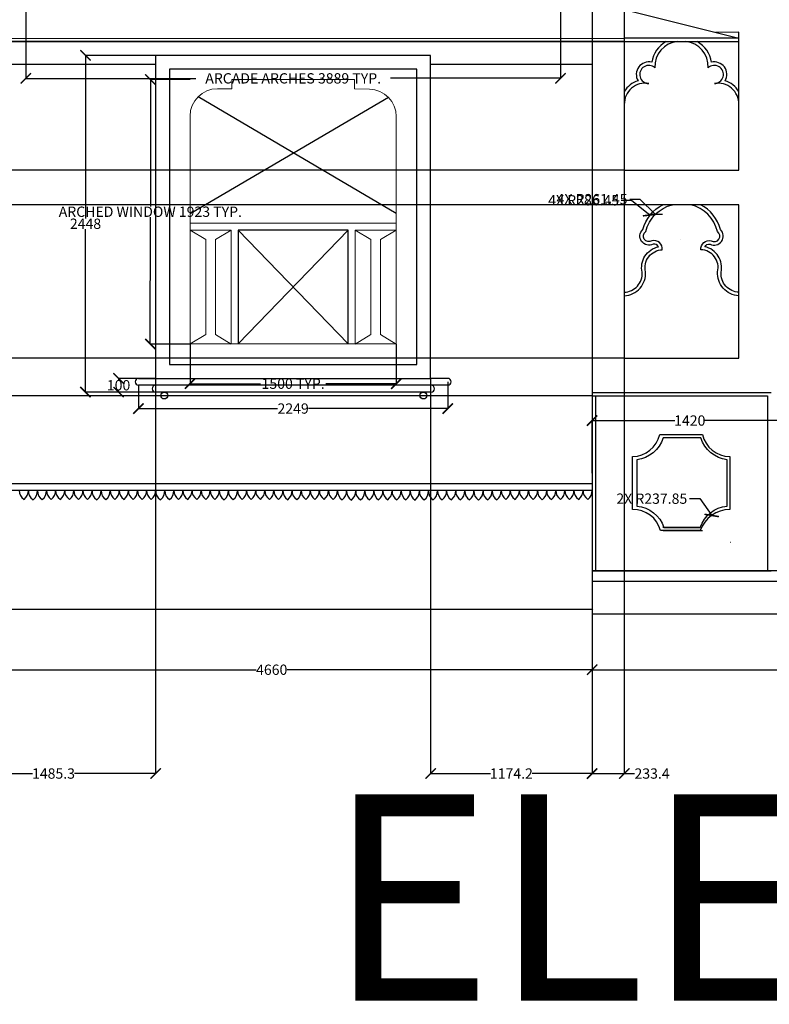
# Model space of a CAD drawing. Units: inches. Extents: x 829 to 33356404, y 1874 to 16983.
# Tile 2 of 9: x 5397 to 10848, y 1874 to 9032. Entities that reach past the tile are written whole.
import ezdxf

# ---------------------------------------------------------------- set-up
doc = ezdxf.new("R2010")
doc.units = ezdxf.units.IN
doc.header["$MEASUREMENT"] = 0
doc.header["$PDMODE"] = 3
for name, color, linetype, lineweight in [('A-ANNO-DIMS', 2, 'Continuous', 18), ('A-ANNO-TEXT', 7, 'Continuous', 25), ('A-ELEV', 7, 'Continuous', 25), ('A-GLAZ', 4, 'Continuous', 18)]:
    doc.layers.add(name, color=color, linetype=linetype, lineweight=lineweight)
doc.styles.get("Standard").update_dxf_attribs({"font": 'arial.ttf'})
doc.dimstyles.get("Standard").update_dxf_attribs({"dimtxt": 75, "dimasz": 75, "dimexe": 0.18, "dimexo": 0.0625, "dimgap": 0.09, "dimtad": 0, "dimtih": 1, "dimtoh": 1, "dimdec": 0, "dimzin": 0, "dimdsep": 46, "dimtxsty": 'Standard', "dimblk": 'ARCHTICK', "dimcen": 0.09, "dimadec": 0, "dimazin": 0, "dimtfac": 1, "dimtdec": 0, "dimtofl": 0, "dimtmove": 0, "dimatfit": 3, "dimfxl": 1, "dimtolj": 1, "dimtzin": 0, "dimarcsym": 0})

# ---------------------------------------------------------------- blocks, each defined once
blk = doc.blocks.new('_ArchTick')
at = {"color": 0, "linetype": 'ByBlock', "const_width": 0.15}
blk.add_lwpolyline([(-0.5, -0.5), (0.5, 0.5)], dxfattribs=at)
blk = doc.blocks.new('*D2')
at = {"layer": 'A-ANNO-DIMS', "color": 0, "lineweight": -2, "transparency": 16777216}
for p, q in [((4899.8, 4746.4), (4899.8, 4306.1)), ((9559.8, 4711.5), (9559.8, 4306.1)), ((4899.8, 4306.3), (7116.3, 4306.3)), ((9559.8, 4306.3), (7343.2, 4306.3))]:
    blk.add_line(p, q, dxfattribs=at)
at = {"layer": 'Defpoints', "color": 0, "transparency": 16777216}
for p in [(4899.8, 4746.5), (9559.8, 4711.5), (9559.8, 4306.3)]:
    blk.add_point(p, dxfattribs=at)
at = {"layer": 'A-ANNO-DIMS', "color": 0, "lineweight": -2, "transparency": 16777216, "xscale": 75, "yscale": 75, "zscale": 75, "rotation": 180}
blk.add_blockref('_ArchTick', (4899.8, 4306.3), dxfattribs=at)
at = {"layer": 'A-ANNO-DIMS', "color": 0, "lineweight": -2, "transparency": 16777216, "xscale": 75, "yscale": 75, "zscale": 75}
blk.add_blockref('_ArchTick', (9559.8, 4306.3), dxfattribs=at)
at = {"layer": 'A-ANNO-DIMS', "color": 0, "transparency": 16777216, "insert": (7229.8, 4306.3), "char_height": 75, "attachment_point": 5}
blk.add_mtext('\\A1;4660', dxfattribs=at)
blk = doc.blocks.new('*D3')
at = {"layer": 'A-ANNO-DIMS', "color": 0, "lineweight": -2, "transparency": 16777216}
for p, q in [((9559.8, 4746.4), (9559.8, 4306.1)), ((17559.8, 4746.4), (17559.8, 4306.1)), ((9559.8, 4306.3), (13447.8, 4306.3)), ((17559.8, 4306.3), (13671.8, 4306.3))]:
    blk.add_line(p, q, dxfattribs=at)
at = {"layer": 'Defpoints', "color": 0, "transparency": 16777216}
for p in [(9559.8, 4746.5), (17559.8, 4746.5), (17559.8, 4306.3)]:
    blk.add_point(p, dxfattribs=at)
at = {"layer": 'A-ANNO-DIMS', "color": 0, "lineweight": -2, "transparency": 16777216, "xscale": 75, "yscale": 75, "zscale": 75, "rotation": 180}
blk.add_blockref('_ArchTick', (9559.8, 4306.3), dxfattribs=at)
at = {"layer": 'A-ANNO-DIMS', "color": 0, "lineweight": -2, "transparency": 16777216, "xscale": 75, "yscale": 75, "zscale": 75}
blk.add_blockref('_ArchTick', (17559.8, 4306.3), dxfattribs=at)
at = {"layer": 'A-ANNO-DIMS', "color": 0, "transparency": 16777216, "insert": (13559.8, 4306.3), "char_height": 75, "attachment_point": 5}
blk.add_mtext('\\A1;8000', dxfattribs=at)
blk = doc.blocks.new('*D17')
at = {"layer": 'A-ANNO-DIMS', "color": 0, "lineweight": -2, "transparency": 16777216}
for p, q in [((9559.8, 5735.5), (9559.8, 6118.2)), ((9559.8, 6118), (10161.4, 6118)), ((10979.9, 6118), (10378.3, 6118)), ((10979.9, 5735.5), (10979.9, 6118.2))]:
    blk.add_line(p, q, dxfattribs=at)
at = {"layer": 'Defpoints', "color": 0, "transparency": 16777216}
for p in [(9559.8, 6118), (9559.8, 5735.5), (10979.9, 5735.5)]:
    blk.add_point(p, dxfattribs=at)
at = {"layer": 'A-ANNO-DIMS', "color": 0, "lineweight": -2, "transparency": 16777216, "xscale": 75, "yscale": 75, "zscale": 75, "rotation": 180}
blk.add_blockref('_ArchTick', (9559.8, 6118), dxfattribs=at)
at = {"layer": 'A-ANNO-DIMS', "color": 0, "lineweight": -2, "transparency": 16777216, "xscale": 75, "yscale": 75, "zscale": 75}
blk.add_blockref('_ArchTick', (10979.9, 6118), dxfattribs=at)
at = {"layer": 'A-ANNO-DIMS', "color": 0, "transparency": 16777216, "insert": (10269.9, 6118), "char_height": 75, "attachment_point": 5}
blk.add_mtext('\\A1;1420', dxfattribs=at)
blk = doc.blocks.new('*D34')
at = {"layer": 'A-ANNO-DIMS', "color": 0, "lineweight": -2, "transparency": 16777216}
for p, q in [((9559.8, 5735.5), (9559.8, 6118.2)), ((9559.8, 6118), (10161.4, 6118)), ((10979.9, 6118), (10378.2, 6118)), ((10979.9, 5735.5), (10979.9, 6118.2))]:
    blk.add_line(p, q, dxfattribs=at)
at = {"layer": 'Defpoints', "color": 0, "transparency": 16777216}
for p in [(10979.9, 6118), (9559.8, 5735.5), (10979.9, 5735.5)]:
    blk.add_point(p, dxfattribs=at)
at = {"layer": 'A-ANNO-DIMS', "color": 0, "lineweight": -2, "transparency": 16777216, "xscale": 75, "yscale": 75, "zscale": 75, "rotation": 180}
blk.add_blockref('_ArchTick', (9559.8, 6118), dxfattribs=at)
at = {"layer": 'A-ANNO-DIMS', "color": 0, "lineweight": -2, "transparency": 16777216, "xscale": 75, "yscale": 75, "zscale": 75}
blk.add_blockref('_ArchTick', (10979.9, 6118), dxfattribs=at)
at = {"layer": 'A-ANNO-DIMS', "color": 0, "transparency": 16777216, "insert": (10269.8, 6118), "char_height": 75, "attachment_point": 5}
blk.add_mtext('\\A1;1420', dxfattribs=at)
blk = doc.blocks.new('*D36')
at = {"layer": 'A-ANNO-DIMS', "color": 0, "lineweight": -2, "transparency": 16777216}
for p, q in [((6261.1, 6374.4), (6261.1, 6204.8)), ((8510.1, 6399.4), (8510.1, 6204.8)), ((6261.1, 6205), (7272.8, 6205)), ((8510.1, 6205), (7498.4, 6205))]:
    blk.add_line(p, q, dxfattribs=at)
at = {"layer": 'Defpoints', "color": 0, "transparency": 16777216}
for p in [(6261.1, 6374.5), (8510.1, 6399.5), (6261.1, 6205)]:
    blk.add_point(p, dxfattribs=at)
at = {"layer": 'A-ANNO-DIMS', "color": 0, "lineweight": -2, "transparency": 16777216, "xscale": 75, "yscale": 75, "zscale": 75, "rotation": 180}
blk.add_blockref('_ArchTick', (6261.1, 6205), dxfattribs=at)
at = {"layer": 'A-ANNO-DIMS', "color": 0, "lineweight": -2, "transparency": 16777216, "xscale": 75, "yscale": 75, "zscale": 75}
blk.add_blockref('_ArchTick', (8510.1, 6205), dxfattribs=at)
at = {"layer": 'A-ANNO-DIMS', "color": 0, "transparency": 16777216, "insert": (7385.6, 6205), "char_height": 75, "attachment_point": 5}
blk.add_mtext('\\A1;2249', dxfattribs=at)
blk = doc.blocks.new('*D37')
at = {"layer": 'A-ANNO-DIMS', "color": 0, "lineweight": -2, "transparency": 16777216}
for p, q in [((6385.5, 6424.5), (6115.9, 6424.5)), ((6116, 6424.5), (6116, 6412.9)), ((6385.5, 6324.5), (6115.9, 6324.5)), ((6116, 6324.5), (6116, 6336.1))]:
    blk.add_line(p, q, dxfattribs=at)
at = {"layer": 'Defpoints', "color": 0, "transparency": 16777216}
for p in [(6385.6, 6424.5), (6116, 6324.5), (6385.6, 6324.5)]:
    blk.add_point(p, dxfattribs=at)
at = {"layer": 'A-ANNO-DIMS', "color": 0, "lineweight": -2, "transparency": 16777216, "xscale": 75, "yscale": 75, "zscale": 75}
for p, rotation in [((6116, 6424.5), 90), ((6116, 6324.5), 270)]:
    blk.add_blockref('_ArchTick', p, dxfattribs=dict(at, rotation=rotation))
at = {"layer": 'A-ANNO-DIMS', "color": 0, "transparency": 16777216, "insert": (6116, 6374.5), "char_height": 75, "attachment_point": 5}
blk.add_mtext('\\A1;100', dxfattribs=at)
blk = doc.blocks.new('*D38')
at = {"layer": 'A-ANNO-DIMS', "color": 0, "lineweight": -2, "transparency": 16777216}
for p, q in [((6385.5, 8772.5), (5875.4, 8772.5)), ((5875.6, 8772.5), (5875.6, 7586.9)), ((5875.6, 6324.5), (5875.6, 7510.1)), ((6385.5, 6324.5), (5875.4, 6324.5))]:
    blk.add_line(p, q, dxfattribs=at)
at = {"layer": 'Defpoints', "color": 0, "transparency": 16777216}
for p in [(6385.6, 8772.5), (5875.6, 6324.5), (6385.6, 6324.5)]:
    blk.add_point(p, dxfattribs=at)
at = {"layer": 'A-ANNO-DIMS', "color": 0, "lineweight": -2, "transparency": 16777216, "xscale": 75, "yscale": 75, "zscale": 75}
for p, rotation in [((5875.6, 8772.5), 90), ((5875.6, 6324.5), 270)]:
    blk.add_blockref('_ArchTick', p, dxfattribs=dict(at, rotation=rotation))
at = {"layer": 'A-ANNO-DIMS', "color": 0, "transparency": 16777216, "insert": (5875.6, 7548.5), "char_height": 75, "attachment_point": 5}
blk.add_mtext('\\A1;2448', dxfattribs=at)
blk = doc.blocks.new('WIN-ARCHED')
for p, q in [((304, 1923.2), (1196, 1923.2)), ((304, 1923.2), (304, 1856.3)), ((1196, 1923.2), (1196, 1856.3)), ((304, 1856.3), (194.7, 1853.4)), ((1196, 1856.3), (1300, 1856.3)), ((0, 0.2), (0, 1653.5)), ((1500, 1656.3), (1500, 0.2)), ((0, 826.9), (300, 827.1)), ((0, 827.1), (115, 759.1)), ((300, 827.1), (185, 759.1)), ((300, 0.2), (300, 827.1)), ((1200, 828), (1500, 828.3)), ((1200, 828.3), (1315, 760.3)), ((1200, 828), (1200, 0.2)), ((1500, 828.3), (1385, 760.3)), ((115, 759.1), (115, 68.1)), ((185, 759.1), (185, 68.1)), ((1315, 760.3), (1315, 68)), ((1385, 760.3), (1385, 68.1)), ((0, 0.1), (115, 68.1)), ((1500, 0.2), (0, 0.2)), ((300, 0.1), (185, 68.1)), ((1200, 0), (1315, 68)), ((1500, 0.1), (1385, 68.1))]:
    blk.add_line(p, q)
for centre, start, end in [((200, 1653.5), 91.52545, 180), ((1300, 1656.3), 0, 90)]:
    blk.add_arc(centre, 200, start, end)
blk = doc.blocks.new('*D78')
at = {"layer": 'A-ANNO-DIMS', "color": 0, "lineweight": -2, "transparency": 16777216}
for p, q in [((6635.6, 8597.5), (6347, 8597.5)), ((6347.1, 8597.5), (6347.1, 7674.8)), ((6347, 6674.3), (6347.1, 7597)), ((6635.4, 6674.3), (6346.8, 6674.3))]:
    blk.add_line(p, q, dxfattribs=at)
at = {"layer": 'Defpoints', "color": 0, "transparency": 16777216}
for p in [(6347.1, 8597.5), (6635.6, 8597.5), (6635.5, 6674.3)]:
    blk.add_point(p, dxfattribs=at)
at = {"layer": 'A-ANNO-DIMS', "color": 0, "lineweight": -2, "transparency": 16777216, "xscale": 75, "yscale": 75, "zscale": 75}
for p, rotation in [((6347.1, 8597.5), 89.99618185466522), ((6347, 6674.3), 269.9961818546653)]:
    blk.add_blockref('_ArchTick', p, dxfattribs=dict(at, rotation=rotation))
at = {"layer": 'A-ANNO-DIMS', "color": 0, "transparency": 16777216, "insert": (6347.1, 7635.9), "char_height": 75, "attachment_point": 5}
blk.add_mtext('\\A1;ARCHED WINDOW 1923 TYP.', dxfattribs=at)
blk = doc.blocks.new('*D79')
at = {"layer": 'A-ANNO-DIMS', "color": 0, "lineweight": -2, "transparency": 16777216}
for p, q in [((6635.5, 6674.2), (6635.5, 6385.6)), ((8135.5, 6674.1), (8135.5, 6385.5)), ((6635.5, 6385.8), (7148.1, 6385.8)), ((8135.5, 6385.7), (7622.9, 6385.7))]:
    blk.add_line(p, q, dxfattribs=at)
at = {"layer": 'Defpoints', "color": 0, "transparency": 16777216}
for p in [(6635.5, 6674.3), (8135.5, 6674.2), (6635.5, 6385.8)]:
    blk.add_point(p, dxfattribs=at)
at = {"layer": 'A-ANNO-DIMS', "color": 0, "lineweight": -2, "transparency": 16777216, "xscale": 75, "yscale": 75, "zscale": 75}
for p, rotation in [((6635.5, 6385.8), 179.9961818546652), ((8135.5, 6385.7), 359.9961818546653)]:
    blk.add_blockref('_ArchTick', p, dxfattribs=dict(at, rotation=rotation))
at = {"layer": 'A-ANNO-DIMS', "color": 0, "transparency": 16777216, "insert": (7385.5, 6385.7), "char_height": 75, "attachment_point": 5}
blk.add_mtext('\\A1;1500 TYP.', dxfattribs=at)
blk = doc.blocks.new('*D80')
at = {"layer": 'A-ANNO-DIMS', "color": 0, "lineweight": -2, "transparency": 16777216}
for p, q in [((5441.3, 9188.4), (5441.4, 8604.9)), ((9330, 9189.3), (9330.2, 8605.9)), ((5441.4, 8605.1), (6677, 8605.4)), ((9330.2, 8606.1), (8094.6, 8605.8))]:
    blk.add_line(p, q, dxfattribs=at)
at = {"layer": 'Defpoints', "color": 0, "transparency": 16777216}
for p in [(5441.3, 9188.4), (9330, 9189.4), (9330.2, 8606.1)]:
    blk.add_point(p, dxfattribs=at)
at = {"layer": 'A-ANNO-DIMS', "color": 0, "lineweight": -2, "transparency": 16777216, "xscale": 75, "yscale": 75, "zscale": 75}
for p, rotation in [((5441.4, 8605.1), 180.0138445878549), ((9330.2, 8606.1), 0.0138445878549074)]:
    blk.add_blockref('_ArchTick', p, dxfattribs=dict(at, rotation=rotation))
at = {"layer": 'A-ANNO-DIMS', "color": 0, "transparency": 16777216, "insert": (7385.8, 8605.6), "char_height": 75, "attachment_point": 5}
blk.add_mtext('\\A1;ARCADE ARCHES 3889 TYP.', dxfattribs=at)
blk = doc.blocks.new('*D83')
at = {"layer": 'A-ANNO-DIMS', "color": 0, "lineweight": -2, "transparency": 16777216}
for p, q in [((13604.5, 15734.9), (985.4, 15734.9)), ((985.6, 15734.9), (985.6, 10279.1)), ((985.6, 4746.5), (985.6, 10202.3)), ((3169.7, 4746.5), (985.4, 4746.5))]:
    blk.add_line(p, q, dxfattribs=at)
at = {"layer": 'Defpoints', "color": 0, "transparency": 16777216}
for p in [(985.6, 15734.9), (13604.5, 15734.9), (3169.8, 4746.5)]:
    blk.add_point(p, dxfattribs=at)
at = {"layer": 'A-ANNO-DIMS', "color": 0, "lineweight": -2, "transparency": 16777216, "xscale": 75, "yscale": 75, "zscale": 75}
for p, rotation in [((985.6, 15734.9), 90), ((985.6, 4746.5), 270)]:
    blk.add_blockref('_ArchTick', p, dxfattribs=dict(at, rotation=rotation))
at = {"layer": 'A-ANNO-DIMS', "color": 0, "transparency": 16777216, "insert": (985.6, 10240.7), "char_height": 75, "attachment_point": 5}
blk.add_mtext('\\A1;10988', dxfattribs=at)
blk = doc.blocks.new('*D86')
at = {"layer": 'A-ANNO-DIMS', "color": 0, "lineweight": -2, "transparency": 16777216}
for p, q in [((4900.3, 6410.1), (4900.3, 3551.3)), ((6385.6, 6424.4), (6385.6, 3551.3)), ((4900.3, 3551.5), (5490.7, 3551.5)), ((6385.6, 3551.5), (5795.2, 3551.5))]:
    blk.add_line(p, q, dxfattribs=at)
at = {"layer": 'Defpoints', "color": 0, "transparency": 16777216}
for p in [(4900.3, 6410.2), (6385.6, 6424.5), (6385.6, 3551.5)]:
    blk.add_point(p, dxfattribs=at)
at = {"layer": 'A-ANNO-DIMS', "color": 0, "lineweight": -2, "transparency": 16777216, "xscale": 75, "yscale": 75, "zscale": 75, "rotation": 180}
blk.add_blockref('_ArchTick', (4900.3, 3551.5), dxfattribs=at)
at = {"layer": 'A-ANNO-DIMS', "color": 0, "lineweight": -2, "transparency": 16777216, "xscale": 75, "yscale": 75, "zscale": 75}
blk.add_blockref('_ArchTick', (6385.6, 3551.5), dxfattribs=at)
at = {"layer": 'A-ANNO-DIMS', "color": 0, "transparency": 16777216, "insert": (5642.9, 3551.5), "char_height": 75, "attachment_point": 5}
blk.add_mtext('\\A1;1485.3', dxfattribs=at)
blk = doc.blocks.new('*D87')
at = {"layer": 'A-ANNO-DIMS', "color": 0, "lineweight": -2, "transparency": 16777216}
for p, q in [((8385.6, 6424.4), (8385.6, 3551.3)), ((9559.8, 6321.4), (9559.8, 3551.3)), ((8385.6, 3551.5), (8820.8, 3551.5)), ((9559.8, 3551.5), (9124.5, 3551.5))]:
    blk.add_line(p, q, dxfattribs=at)
at = {"layer": 'Defpoints', "color": 0, "transparency": 16777216}
for p in [(8385.6, 6424.5), (9559.8, 6321.5), (9559.8, 3551.5)]:
    blk.add_point(p, dxfattribs=at)
at = {"layer": 'A-ANNO-DIMS', "color": 0, "lineweight": -2, "transparency": 16777216, "xscale": 75, "yscale": 75, "zscale": 75, "rotation": 180}
blk.add_blockref('_ArchTick', (8385.6, 3551.5), dxfattribs=at)
at = {"layer": 'A-ANNO-DIMS', "color": 0, "lineweight": -2, "transparency": 16777216, "xscale": 75, "yscale": 75, "zscale": 75}
blk.add_blockref('_ArchTick', (9559.8, 3551.5), dxfattribs=at)
at = {"layer": 'A-ANNO-DIMS', "color": 0, "transparency": 16777216, "insert": (8972.7, 3551.5), "char_height": 75, "attachment_point": 5}
blk.add_mtext('\\A1;1174.2', dxfattribs=at)
blk = doc.blocks.new('*D94')
at = {"layer": 'A-ANNO-DIMS', "color": 0, "lineweight": -2, "transparency": 16777216}
for p, q in [((9793.9, 6572.4), (985.4, 6572.4)), ((985.6, 6572.4), (985.6, 6472.8)), ((985.6, 6296.5), (985.6, 6396.1)), ((9559.7, 6296.5), (985.4, 6296.5))]:
    blk.add_line(p, q, dxfattribs=at)
at = {"layer": 'Defpoints', "color": 0, "transparency": 16777216}
for p in [(985.6, 6572.4), (9793.9, 6572.4), (9559.8, 6296.5)]:
    blk.add_point(p, dxfattribs=at)
at = {"layer": 'A-ANNO-DIMS', "color": 0, "lineweight": -2, "transparency": 16777216, "xscale": 75, "yscale": 75, "zscale": 75}
for p, rotation in [((985.6, 6572.4), 90), ((985.6, 6296.5), 270)]:
    blk.add_blockref('_ArchTick', p, dxfattribs=dict(at, rotation=rotation))
at = {"layer": 'A-ANNO-DIMS', "color": 0, "transparency": 16777216, "insert": (985.6, 6434.5), "char_height": 75, "attachment_point": 5}
blk.add_mtext('\\A1;275.97', dxfattribs=at)
blk = doc.blocks.new('*D95')
at = {"layer": 'A-ANNO-DIMS', "color": 0, "lineweight": -2, "transparency": 16777216}
for p, q in [((9793.9, 7687.3), (985.4, 7687.3)), ((985.6, 7687.3), (985.6, 7168.2)), ((985.6, 6572.4), (985.6, 7091.5)), ((9793.9, 6572.4), (985.4, 6572.4))]:
    blk.add_line(p, q, dxfattribs=at)
at = {"layer": 'Defpoints', "color": 0, "transparency": 16777216}
for p in [(985.6, 7687.3), (9793.9, 7687.3), (9793.9, 6572.4)]:
    blk.add_point(p, dxfattribs=at)
at = {"layer": 'A-ANNO-DIMS', "color": 0, "lineweight": -2, "transparency": 16777216, "xscale": 75, "yscale": 75, "zscale": 75}
for p, rotation in [((985.6, 7687.3), 90), ((985.6, 6572.4), 270)]:
    blk.add_blockref('_ArchTick', p, dxfattribs=dict(at, rotation=rotation))
at = {"layer": 'A-ANNO-DIMS', "color": 0, "transparency": 16777216, "insert": (985.6, 7129.8), "char_height": 75, "attachment_point": 5}
blk.add_mtext('\\A1;1114.8', dxfattribs=at)
blk = doc.blocks.new('*D96')
at = {"layer": 'A-ANNO-DIMS', "color": 0, "lineweight": -2, "transparency": 16777216}
for p, q in [((9793.7, 7937.3), (985.4, 7937.3)), ((985.6, 7937.3), (985.6, 7850.6)), ((985.6, 7687.3), (985.6, 7773.9)), ((9793.9, 7687.3), (985.4, 7687.3))]:
    blk.add_line(p, q, dxfattribs=at)
at = {"layer": 'Defpoints', "color": 0, "transparency": 16777216}
for p in [(985.6, 7937.3), (9793.7, 7937.3), (9793.9, 7687.3)]:
    blk.add_point(p, dxfattribs=at)
at = {"layer": 'A-ANNO-DIMS', "color": 0, "lineweight": -2, "transparency": 16777216, "xscale": 75, "yscale": 75, "zscale": 75}
for p, rotation in [((985.6, 7937.3), 90), ((985.6, 7687.3), 270)]:
    blk.add_blockref('_ArchTick', p, dxfattribs=dict(at, rotation=rotation))
at = {"layer": 'A-ANNO-DIMS', "color": 0, "transparency": 16777216, "insert": (985.6, 7812.3), "char_height": 75, "attachment_point": 5}
blk.add_mtext('\\A1;250', dxfattribs=at)
blk = doc.blocks.new('*D97')
at = {"layer": 'A-ANNO-DIMS', "color": 0, "lineweight": -2, "transparency": 16777216}
for p, q in [((9793.7, 8872.5), (985.4, 8872.5)), ((985.6, 8872.5), (985.6, 8443.3)), ((985.6, 7937.3), (985.6, 8366.5)), ((9793.7, 7937.3), (985.4, 7937.3))]:
    blk.add_line(p, q, dxfattribs=at)
at = {"layer": 'Defpoints', "color": 0, "transparency": 16777216}
for p in [(985.6, 8872.5), (9793.7, 8872.5), (9793.7, 7937.3)]:
    blk.add_point(p, dxfattribs=at)
at = {"layer": 'A-ANNO-DIMS', "color": 0, "lineweight": -2, "transparency": 16777216, "xscale": 75, "yscale": 75, "zscale": 75}
for p, rotation in [((985.6, 8872.5), 90), ((985.6, 7937.3), 270)]:
    blk.add_blockref('_ArchTick', p, dxfattribs=dict(at, rotation=rotation))
at = {"layer": 'A-ANNO-DIMS', "color": 0, "transparency": 16777216, "insert": (985.6, 8404.9), "char_height": 75, "attachment_point": 5}
blk.add_mtext('\\A1;935.2', dxfattribs=at)
blk = doc.blocks.new('*D98')
at = {"layer": 'A-ANNO-DIMS', "color": 0, "lineweight": -2, "transparency": 16777216}
for p, q in [((9793.7, 9165.5), (985.4, 9165.5)), ((985.6, 9165.5), (985.6, 9057.4)), ((985.6, 8872.5), (985.6, 8980.6)), ((9793.7, 8872.5), (985.4, 8872.5))]:
    blk.add_line(p, q, dxfattribs=at)
at = {"layer": 'Defpoints', "color": 0, "transparency": 16777216}
for p in [(985.6, 9165.5), (9793.7, 9165.5), (9793.7, 8872.5)]:
    blk.add_point(p, dxfattribs=at)
at = {"layer": 'A-ANNO-DIMS', "color": 0, "lineweight": -2, "transparency": 16777216, "xscale": 75, "yscale": 75, "zscale": 75}
for p, rotation in [((985.6, 9165.5), 90), ((985.6, 8872.5), 270)]:
    blk.add_blockref('_ArchTick', p, dxfattribs=dict(at, rotation=rotation))
at = {"layer": 'A-ANNO-DIMS', "color": 0, "transparency": 16777216, "insert": (985.6, 9019), "char_height": 75, "attachment_point": 5}
blk.add_mtext('\\A1;293', dxfattribs=at)
blk = doc.blocks.new('*D108')
at = {"layer": 'A-ANNO-DIMS', "color": 0, "lineweight": -2, "transparency": 16777216}
for p, q in [((9560.3, 9165.4), (9560.3, 3551.3)), ((9793.7, 9165.4), (9793.7, 3551.3)), ((9560.3, 3551.5), (9793.7, 3551.5)), ((9793.7, 3551.5), (9868.7, 3551.5))]:
    blk.add_line(p, q, dxfattribs=at)
at = {"layer": 'Defpoints', "color": 0, "transparency": 16777216}
for p in [(9560.3, 9165.5), (9793.7, 9165.5), (9793.7, 3551.5)]:
    blk.add_point(p, dxfattribs=at)
at = {"layer": 'A-ANNO-DIMS', "color": 0, "lineweight": -2, "transparency": 16777216, "xscale": 75, "yscale": 75, "zscale": 75, "rotation": 180}
blk.add_blockref('_ArchTick', (9560.3, 3551.5), dxfattribs=at)
at = {"layer": 'A-ANNO-DIMS', "color": 0, "lineweight": -2, "transparency": 16777216, "xscale": 75, "yscale": 75, "zscale": 75}
blk.add_blockref('_ArchTick', (9793.7, 3551.5), dxfattribs=at)
at = {"layer": 'A-ANNO-DIMS', "color": 0, "transparency": 16777216, "insert": (9995.8, 3551.5), "char_height": 75, "attachment_point": 5}
blk.add_mtext('\\A1;233.4', dxfattribs=at)
blk = doc.blocks.new('*D131')
at = {"layer": 'A-ANNO-DIMS', "color": 0, "lineweight": -2, "transparency": 16777216}
for p, q in [((9772.2, 7719.3), (9847.2, 7719.3)), ((9847.2, 7719.3), (9981.4, 7612)), ((10205.1, 7433.1), (10205.3, 7433.1)), ((10205.2, 7433), (10205.2, 7433.2))]:
    blk.add_line(p, q, dxfattribs=at)
at = {"layer": 'Defpoints', "color": 0, "transparency": 16777216}
for p in [(9981.4, 7612), (10205.2, 7433.1)]:
    blk.add_point(p, dxfattribs=at)
at = {"layer": 'A-ANNO-DIMS', "color": 0, "lineweight": -2, "transparency": 16777216, "xscale": 75, "yscale": 75, "zscale": 75, "rotation": 321.3591378305642}
blk.add_blockref('_ArchTick', (9981.4, 7612), dxfattribs=at)
at = {"layer": 'A-ANNO-DIMS', "color": 0, "transparency": 16777216, "insert": (9498.2, 7719.3), "char_height": 75, "attachment_point": 5}
blk.add_mtext('\\A1;4X R286.45', dxfattribs=at)
blk = doc.blocks.new('*D132')
at = {"layer": 'A-ANNO-DIMS', "color": 0, "lineweight": -2, "transparency": 16777216}
for p, q in [((9832.9, 7727.4), (9907.9, 7727.4)), ((9907.9, 7727.4), (10019.4, 7617.1)), ((10205.1, 7433.1), (10205.3, 7433.1)), ((10205.2, 7433), (10205.2, 7433.2))]:
    blk.add_line(p, q, dxfattribs=at)
at = {"layer": 'Defpoints', "color": 0, "transparency": 16777216}
for p in [(10019.4, 7617.1), (10205.2, 7433.1)]:
    blk.add_point(p, dxfattribs=at)
at = {"layer": 'A-ANNO-DIMS', "color": 0, "lineweight": -2, "transparency": 16777216, "xscale": 75, "yscale": 75, "zscale": 75, "rotation": 315.2866369533732}
blk.add_blockref('_ArchTick', (10019.4, 7617.1), dxfattribs=at)
at = {"layer": 'A-ANNO-DIMS', "color": 0, "transparency": 16777216, "insert": (9558.9, 7727.4), "char_height": 75, "attachment_point": 5}
blk.add_mtext('\\A1;4X R261.45', dxfattribs=at)
blk = doc.blocks.new('*D136')
at = {"layer": 'A-ANNO-DIMS', "color": 0, "lineweight": -2, "transparency": 16777216}
for p, q in [((10267, 5549.9), (10342, 5549.9)), ((10342, 5549.9), (10429.2, 5427.8)), ((10567.3, 5234.2), (10567.4, 5234.2)), ((10567.4, 5234.1), (10567.4, 5234.3))]:
    blk.add_line(p, q, dxfattribs=at)
at = {"layer": 'Defpoints', "color": 0, "transparency": 16777216}
for p in [(10429.2, 5427.8), (10567.4, 5234.2)]:
    blk.add_point(p, dxfattribs=at)
at = {"layer": 'A-ANNO-DIMS', "color": 0, "lineweight": -2, "transparency": 16777216, "xscale": 75, "yscale": 75, "zscale": 75, "rotation": 305.5232203539446}
blk.add_blockref('_ArchTick', (10429.2, 5427.8), dxfattribs=at)
at = {"layer": 'A-ANNO-DIMS', "color": 0, "transparency": 16777216, "insert": (9993.8, 5549.9), "char_height": 75, "attachment_point": 5}
blk.add_mtext('\\A1;2X R237.85', dxfattribs=at)

msp = doc.modelspace()

# ---------------------------------------------------------------- linework, layer by layer
at = {"layer": 'A-ELEV'}
for p, q in [((9560.336, 9165.468), (10626.905, 8897.385)), ((3802.555, 8894.205), (9793.728, 8897.385)), ((10626.905, 8940.247), (10456.855, 8940.128)), ((10626.905, 8897.385), (10626.905, 8940.247)), ((3784.24, 8872.468), (10626.905, 8872.468)), ((6385.56, 8772.468), (6385.56, 6424.468)), ((8385.56, 8772.468), (6385.56, 8772.468)), ((8385.56, 6424.468), (8385.56, 8772.468)), ((4900.278, 8708.468), (6385.56, 8708.468)), ((8385.56, 8708.468), (9560.278, 8708.468)), ((9560.278, 8708.468), (9559.893, 5660.468)), ((8078.851, 8467.25), (6635.56, 7621.325)), ((8135.56, 7623.901), (6694.138, 8471.984)), ((8135.607, 7551.096), (6635.607, 7552.516)), ((6885.56, 7552.326), (6885.56, 7552.279)), ((6820.56, 7502.397), (6820.56, 7502.37)), ((6985.56, 7502.232), (6985.56, 6674.468)), ((7785.56, 7501.38), (6985.56, 7501.38)), ((6985.56, 7501.38), (7785.56, 6674.468)), ((6985.56, 6674.468), (7785.56, 7501.38)), ((7785.56, 6674.468), (7785.56, 7501.38)), ((8020.56, 7501.214), (8020.56, 7501.187)), ((6261.06, 6424.468), (6385.56, 6424.468)), ((8510.06, 6374.468), (6261.06, 6374.468)), ((6385.56, 6424.468), (8385.56, 6424.468)), ((8510.06, 6424.468), (8385.56, 6424.468)), ((8388.085, 6324.468), (6385.56, 6324.468)), ((9559.807, 6321.468), (10860.89, 6321.304)), ((9559.804, 6296.468), (10835.89, 6296.307)), ((9584.778, 6296.307), (9584.778, 5024.468)), ((10835.89, 6296.307), (10835.89, 5024.468)), ((3119.778, 5660.468), (9559.893, 5660.468)), ((3119.778, 5610.468), (9559.887, 5610.468)), ((9559.887, 5610.468), (9559.778, 4746.468)), ((9559.692, 5024.468), (10860.89, 5024.468)), ((10979.778, 5024.468), (9559.778, 5024.468)), ((9559.778, 4949.468), (17559.778, 4949.468)), ((4899.778, 4746.468), (9559.778, 4746.468)), ((9275.666, 4746.468), (9275.666, 4746.267)), ((9350.666, 4746.468), (9350.666, 4746.276)), ((9450.666, 4746.468), (9450.666, 4746.289)), ((9569.666, 4746.468), (9569.666, 4746.304)), ((9559.778, 4711.528), (17559.778, 4711.528))]:
    msp.add_line(p, q, dxfattribs=at)
for points in [[(9793.728, 8872.468), (9793.728, 7937.261), (10626.905, 7937.261), (10626.905, 8897.385), (9793.728, 8897.385)], [(10344.691, 5317.852), (10057.889, 5317.468)], [(10338.649, 5340.542), (10074.47, 5340.542)], [(10075.978, 5317.852), (10362.779, 5317.468)], [(10082.019, 5340.542), (10346.198, 5340.542)]]:
    msp.add_lwpolyline(points, dxfattribs=at)
for points in [[(10181.89, 8872.468, 0.40989122), (10017.024, 8682.012, 1.47300783), (9971.853, 8568.249, 0.47165222), (9793.728, 8416.104)], [(10097.11, 8872.468, 0.23532644), (9993.676, 8722.287, 0.66528938), (9893.689, 8587.794, 0.18580943), (9793.728, 8509.437, 0.18580943)], [(10448.78, 8568.249, 1.47300783), (10403.609, 8682.012, 0.40989122), (10238.744, 8872.468)], [(10526.944, 8587.794, 0.66528938), (10426.957, 8722.287, 0.23532644), (10323.523, 8872.468, 0.23532644)], [(9792.781, 7049.962, 0.41856692), (9923.733, 7195.519, -0.41804495), (10041.692, 7381.328, 0.32232847), (10003.632, 7401.223, -0.8791924), (9928.168, 7506.037, -0.21156079), (10073.05, 7687.262, -0.21156079)], [(9793.914, 7024.987), (9793.914, 7024.987, 0.42265931), (9948.536, 7199.277, -0.47714562), (10070.397, 7359.767, 0.50944673), (9994.634, 7424.938, -0.99585069), (9950.42, 7491.881, -0.28412367), (10143.857, 7687.262)], [(10627.092, 7024.987), (10627.092, 7024.987, -0.42265931), (10472.471, 7199.277, 0.47714562), (10350.609, 7359.767, -0.50944673), (10426.373, 7424.938, 0.99585069), (10470.586, 7491.881, 0.28412367), (10277.15, 7687.262)], [(10628.225, 7049.962, -0.41856692), (10497.274, 7195.519, 0.41804495), (10379.314, 7381.328, -0.32232847), (10417.375, 7401.223, 0.8791924), (10492.839, 7506.037, 0.21156079), (10347.957, 7687.262, 0.21156079)], [(10057.889, 5317.468, 0.3413811), (9853.869, 5471.984), (9853.869, 5856.29, 0.3446138), (10052.118, 6015.968), (10362.342, 6015.968, 0.3446138), (10560.591, 5856.29), (10560.591, 5471.984, 0.30471722), (10344.691, 5317.852, 0.32430238)], [(10346.198, 5340.542, -0.29882249), (10541.8, 5495.944), (10541.8, 5832.963, -0.29137991), (10349.6, 5990.968), (10077.277, 5990.968, -0.29137991), (9885.078, 5832.963), (9885.078, 5495.944, -0.29428256), (10082.029, 5340.513)], [(5393.91, 5610.468, 0.26781097), (5428.368, 5544.592, 0.24469844), (5460, 5610.468, 0.24469844)], [(5460.041, 5610.468, 0.27512595), (5494.498, 5542.037, 0.25167024), (5526.13, 5610.468, 0.24469844)], [(5526.202, 5609.062, 0.26781097), (5560.66, 5543.186, 0.24469844), (5592.292, 5609.062, 0.24469844)], [(5592.392, 5610.468, 0.26781097), (5626.849, 5544.592, 0.24469844), (5658.481, 5610.468, 0.24469844)], [(5658.392, 5610.463, 0.26781097), (5692.85, 5544.587, 0.24469844), (5724.482, 5610.463, 0.24469844)], [(5724.585, 5610.468, 0.26781097), (5759.042, 5544.592, 0.24469844), (5790.674, 5610.468, 0.24469844)], [(5790.674, 5610.468, 0.26781097), (5825.132, 5544.592, 0.24469844), (5856.764, 5610.468, 0.24469844)], [(5856.764, 5610.468, 0.26781097), (5891.221, 5544.592, 0.24469844), (5922.853, 5610.468, 0.24469844)], [(5922.894, 5610.468, 0.27512595), (5957.351, 5542.037, 0.25167024), (5988.984, 5610.468, 0.24469844)], [(5989.056, 5609.062, 0.26781097), (6023.513, 5543.186, 0.24469844), (6055.145, 5609.062, 0.24469844)], [(6055.245, 5610.468, 0.26781097), (6089.702, 5544.592, 0.24469844), (6121.334, 5610.468, 0.24469844)], [(6121.246, 5610.463, 0.26781097), (6155.703, 5544.587, 0.24469844), (6187.335, 5610.463, 0.24469844)], [(6187.438, 5610.468, 0.26781097), (6221.896, 5544.592, 0.24469844), (6253.528, 5610.468, 0.24469844)], [(6253.528, 5610.468, 0.26781097), (6287.985, 5544.592, 0.24469844), (6319.617, 5610.468, 0.24469844)], [(6319.681, 5610.468, 0.26781097), (6354.138, 5544.592, 0.24469844), (6385.77, 5610.468, 0.24469844)], [(6385.811, 5610.468, 0.27512595), (6420.269, 5542.037, 0.25167024), (6451.901, 5610.468, 0.24469844)], [(6451.973, 5609.062, 0.26781097), (6486.43, 5543.186, 0.24469844), (6518.062, 5609.062, 0.24469844)], [(6518.162, 5610.468, 0.26781097), (6552.62, 5544.592, 0.24469844), (6584.252, 5610.468, 0.24469844)], [(6584.163, 5610.463, 0.26781097), (6618.62, 5544.587, 0.24469844), (6650.252, 5610.463, 0.24469844)], [(6650.356, 5610.468, 0.26781097), (6684.813, 5544.592, 0.24469844), (6716.445, 5610.468, 0.24469844)], [(6716.445, 5610.468, 0.26781097), (6750.902, 5544.592, 0.24469844), (6782.534, 5610.468, 0.24469844)], [(6782.534, 5610.468, 0.26781097), (6816.991, 5544.592, 0.24469844), (6848.624, 5610.468, 0.24469844)], [(6848.665, 5610.468, 0.27512595), (6883.122, 5542.037, 0.25167024), (6914.754, 5610.468, 0.24469844)], [(6914.826, 5609.062, 0.26781097), (6949.284, 5543.186, 0.24469844), (6980.916, 5609.062, 0.24469844)], [(6981.016, 5610.468, 0.26781097), (7015.473, 5544.592, 0.24469844), (7047.105, 5610.468, 0.24469844)], [(7047.016, 5610.463, 0.26781097), (7081.474, 5544.587, 0.24469844), (7113.106, 5610.463, 0.24469844)], [(7113.209, 5610.468, 0.26781097), (7147.666, 5544.592, 0.24469844), (7179.298, 5610.468, 0.24469844)], [(7179.298, 5610.468, 0.26781097), (7213.756, 5544.592, 0.24469844), (7245.388, 5610.468, 0.24469844)], [(7245.451, 5610.468, 0.26781097), (7279.909, 5544.592, 0.24469844), (7311.541, 5610.468, 0.24469844)], [(7311.582, 5610.468, 0.27512595), (7346.039, 5542.037, 0.25167024), (7377.671, 5610.468, 0.24469844)], [(7377.743, 5609.062, 0.26781097), (7412.201, 5543.186, 0.24469844), (7443.833, 5609.062, 0.24469844)], [(7443.933, 5610.468, 0.26781097), (7478.39, 5544.592, 0.24469844), (7510.022, 5610.468, 0.24469844)], [(7509.934, 5610.463, 0.26781097), (7544.391, 5544.587, 0.24469844), (7576.023, 5610.463, 0.24469844)], [(7576.126, 5610.468, 0.26781097), (7610.583, 5544.592, 0.24469844), (7642.215, 5610.468, 0.24469844)], [(7642.215, 5610.468, 0.26781097), (7676.673, 5544.592, 0.24469844), (7708.305, 5610.468, 0.24469844)], [(7708.346, 5607.838, 0.26781097), (7742.803, 5541.962, 0.24469844), (7774.435, 5607.838, 0.24469844)], [(7774.477, 5607.838, 0.27512595), (7808.934, 5539.406, 0.25167024), (7840.566, 5607.838, 0.24469844)], [(7840.638, 5606.431, 0.26781097), (7875.095, 5540.555, 0.24469844), (7906.727, 5606.431, 0.24469844)], [(7906.828, 5607.838, 0.26781097), (7941.285, 5541.962, 0.24469844), (7972.917, 5607.838, 0.24469844)], [(7972.828, 5607.832, 0.26781097), (8007.285, 5541.956, 0.24469844), (8038.917, 5607.832, 0.24469844)], [(8039.021, 5607.838, 0.26781097), (8073.478, 5541.962, 0.24469844), (8105.11, 5607.838, 0.24469844)], [(8105.11, 5607.838, 0.26781097), (8139.567, 5541.962, 0.24469844), (8171.199, 5607.838, 0.24469844)], [(8171.263, 5607.838, 0.26781097), (8205.72, 5541.962, 0.24469844), (8237.353, 5607.838, 0.24469844)], [(8237.394, 5607.838, 0.27512595), (8271.851, 5539.406, 0.25167024), (8303.483, 5607.838, 0.24469844)], [(8303.555, 5606.431, 0.26781097), (8338.013, 5540.555, 0.24469844), (8369.645, 5606.431, 0.24469844)], [(8369.745, 5607.838, 0.26781097), (8404.202, 5541.962, 0.24469844), (8435.834, 5607.838, 0.24469844)], [(8435.745, 5607.832, 0.26781097), (8470.203, 5541.956, 0.24469844), (8501.835, 5607.832, 0.24469844)], [(8501.938, 5607.838, 0.26781097), (8536.395, 5541.962, 0.24469844), (8568.027, 5607.838, 0.24469844)], [(8568.027, 5607.838, 0.26781097), (8602.485, 5541.962, 0.24469844), (8634.117, 5607.838, 0.24469844)], [(8634.117, 5607.838, 0.26781097), (8668.574, 5541.962, 0.24469844), (8700.206, 5607.838, 0.24469844)], [(8700.247, 5607.838, 0.27512595), (8734.704, 5539.406, 0.25167024), (8766.336, 5607.838, 0.24469844)], [(8766.409, 5606.431, 0.26781097), (8800.866, 5540.555, 0.24469844), (8832.498, 5606.431, 0.24469844)], [(8832.598, 5607.838, 0.26781097), (8867.055, 5541.962, 0.24469844), (8898.687, 5607.838, 0.24469844)], [(8898.599, 5610.463, 0.26781097), (8933.056, 5544.587, 0.24469844), (8964.688, 5610.463, 0.24469844)], [(8964.791, 5610.468, 0.26781097), (8999.249, 5544.592, 0.24469844), (9030.881, 5610.468, 0.24469844)], [(9030.881, 5610.468, 0.26781097), (9065.338, 5544.592, 0.24469844), (9096.97, 5610.468, 0.24469844)], [(9097.034, 5610.468, 0.26781097), (9131.491, 5544.592, 0.24469844), (9163.123, 5610.468, 0.24469844)], [(9163.164, 5610.468, 0.27512595), (9197.622, 5542.037, 0.25167024), (9229.254, 5610.468, 0.24469844)], [(9229.326, 5609.062, 0.26781097), (9263.783, 5543.186, 0.24469844), (9295.415, 5609.062, 0.24469844)], [(9295.515, 5610.468, 0.26781097), (9329.973, 5544.592, 0.24469844), (9361.605, 5610.468, 0.24469844)], [(9361.516, 5610.463, 0.26781097), (9395.973, 5544.587, 0.24469844), (9427.605, 5610.463, 0.24469844)], [(9427.709, 5610.468, 0.26781097), (9462.166, 5544.592, 0.24469844), (9493.798, 5610.468, 0.24469844)], [(9493.798, 5610.468, 0.26781097), (9528.255, 5544.592, 0.24469844), (9559.887, 5610.468, 0.24469844)]]:
    msp.add_lwpolyline(points, format="xyb", dxfattribs=at)
for points in [[(6485.56, 8672.468), (6485.56, 6524.468), (8285.56, 6524.468), (8285.56, 8672.468)], [(10627.092, 7687.262), (9793.914, 7687.262), (9793.914, 6572.436), (10627.092, 6572.436)]]:
    msp.add_lwpolyline(points, close=True, dxfattribs=at)
for centre in [(6448.692, 6299.468), (8332.731, 6299.468)]:
    msp.add_circle(centre, 25, dxfattribs=at)
for centre, radius, start, end in [((10475.138, 8418.764), 151.79, 358.9959504, 100), ((10475.138, 8418.764), 176.79, 30.8561446, 72.9603597), ((6261.06, 6399.468), 25, 90, 270), ((6385.56, 6349.468), 25, 90, 270), ((8388.085, 6349.468), 25, 270, 90), ((8510.06, 6399.468), 25, 270, 90)]:
    msp.add_arc(centre, radius, start, end, dxfattribs=at)

# ---------------------------------------------------------------- block references
at = {"layer": 'A-GLAZ', "extrusion": (0, 0, -1), "zscale": -1, "rotation": 0.0038181453347709}
msp.add_blockref('WIN-ARCHED', (-8135.501, 6674.182), dxfattribs=at)

# ---------------------------------------------------------------- texts
at = {"layer": 'A-ANNO-TEXT'}
msp.add_text('ELEVATION', height=1500, dxfattribs=at).set_placement((7631.721, 1900.346))

# ---------------------------------------------------------------- dimensions: what is measured, and where the dimension line sits
at = {"layer": 'A-ANNO-DIMS'}
for base, p1, p2, angle, override, picture, middle in [((985.628, 15734.879), (3169.778, 4746.468), (13604.527, 15734.879), 90, {"dimdec": 0, "dimlfac": 1, "dimrnd": 0, "dimzin": 0, "dimdsep": 46, "dimlunit": 2}, '*D83', (985.628, 10240.673)), ((985.628, 9165.468), (9793.728, 8872.468), (9793.728, 9165.468), 90, {"dimdec": 0, "dimlfac": 1, "dimrnd": 0, "dimzin": 0, "dimdsep": 46, "dimlunit": 2}, '*D98', (985.628, 9018.968)), ((985.628, 8872.468), (9793.728, 7937.261), (9793.728, 8872.468), 90, {"dimdec": 1, "dimlfac": 1, "dimrnd": 0, "dimzin": 0, "dimdsep": 46, "dimlunit": 2}, '*D97', (985.628, 8404.865)), ((985.628, 7937.261), (9793.914, 7687.262), (9793.728, 7937.261), 90, {"dimdec": 0, "dimlfac": 1, "dimrnd": 0, "dimzin": 0, "dimdsep": 46, "dimlunit": 2}, '*D96', (985.628, 7812.261)), ((985.628, 7687.262), (9793.914, 6572.436), (9793.914, 7687.262), 90, {"dimdec": 1, "dimlfac": 1, "dimrnd": 0, "dimzin": 0, "dimdsep": 46, "dimlunit": 2}, '*D95', (985.628, 7129.849)), ((985.628, 6572.436), (9559.804, 6296.468), (9793.914, 6572.436), 90, {"dimdec": 2, "dimlfac": 1, "dimrnd": 0, "dimzin": 0, "dimdsep": 46, "dimlunit": 2}, '*D94', (985.628, 6434.452)), ((6261.06, 6205.007), (8510.06, 6399.468), (6261.06, 6374.468), 180, {"dimclrd": 0, "dimclre": 0, "dimclrt": 0}, '*D36', (7385.56, 6205.007)), ((10979.871, 6118.028), (9559.778, 5735.468), (10979.871, 5735.461), 180, {"dimclrd": 0, "dimclre": 0, "dimclrt": 0}, '*D34', (10269.825, 6118.028))]:
    dim = msp.add_linear_dim(base=base, p1=p1, p2=p2, angle=angle, dimstyle='Standard', override=override, dxfattribs=at)
    dim.commit()
    dim.dimension.update_dxf_attribs({"geometry": picture, "text_midpoint": middle})
for base, p1, p2, angle, text, picture, middle in [((9330.166, 8606.059), (5441.282, 9188.431), (9330.025, 9189.371), 0.0138446, 'ARCADE ARCHES <> TYP.', '*D80', (7385.795, 8605.59)), ((6347.144, 8597.537), (6635.501, 6674.282), (6635.629, 8597.518), 89.9961819, 'ARCHED WINDOW <> TYP.', '*D78', (6347.08, 7635.919)), ((6635.482, 6385.796), (8135.501, 6674.182), (6635.501, 6674.282), 179.9961819, '<> TYP.', '*D79', (7385.482, 6385.746))]:
    dim = msp.add_linear_dim(base=base, p1=p1, p2=p2, angle=angle, text=text, dimstyle='Standard', override={"dimdec": 0, "dimrnd": 0, "dimzin": 0, "dimlunit": 2}, dxfattribs=at)
    dim.commit()
    dim.dimension.update_dxf_attribs({"geometry": picture, "text_midpoint": middle})
for base, p1, p2, override, picture, middle in [((9793.728, 3551.528), (9560.336, 9165.468), (9793.728, 9165.468), {"dimdec": 1, "dimlfac": 1, "dimrnd": 0, "dimzin": 0, "dimdsep": 46, "dimlunit": 2}, '*D108', (9995.847, 3551.528)), ((6385.56, 3551.528), (4900.278, 6410.159), (6385.56, 6424.468), {"dimdec": 1, "dimlfac": 1, "dimrnd": 0, "dimzin": 0, "dimdsep": 46, "dimlunit": 2}, '*D86', (5642.919, 3551.528)), ((9559.807, 3551.528), (8385.56, 6424.468), (9559.807, 6321.468), {"dimdec": 1, "dimlfac": 1, "dimrnd": 0, "dimzin": 0, "dimdsep": 46, "dimlunit": 2}, '*D87', (8972.683, 3551.528)), ((9559.81, 6118.028), (10979.903, 5735.468), (9559.81, 5735.461), {"dimclrd": 0, "dimclre": 0, "dimclrt": 0}, '*D17', (10269.856, 6118.028)), ((9559.778, 4306.306), (4899.778, 4746.468), (9559.778, 4711.528), {"dimclrd": 0, "dimclre": 0, "dimclrt": 0}, '*D2', (7229.778, 4306.306)), ((17559.778, 4306.306), (9559.778, 4746.468), (17559.778, 4746.468), {"dimclrd": 0, "dimclre": 0, "dimclrt": 0}, '*D3', (13559.778, 4306.306))]:
    dim = msp.add_linear_dim(base=base, p1=p1, p2=p2, dimstyle='Standard', override=override, dxfattribs=at)
    dim.commit()
    dim.dimension.update_dxf_attribs({"geometry": picture, "text_midpoint": middle})
for base, p1, picture, middle in [((5875.588, 6324.468), (6385.56, 8772.468), '*D38', (5875.588, 7548.468)), ((6116.031, 6324.468), (6385.56, 6424.468), '*D37', (6116.031, 6374.468))]:
    dim = msp.add_linear_dim(base=base, p1=p1, p2=(6385.56, 6324.468), angle=90, dimstyle='Standard', override={"dimclrd": 0, "dimclre": 0, "dimclrt": 0}, dxfattribs=at)
    dim.commit()
    dim.dimension.update_dxf_attribs({"geometry": picture, "text_midpoint": middle, "dimtype": 160})
for mpoint, picture, middle in [((9981.439, 7611.975), '*D131', (9498.172, 7719.296)), ((10019.382, 7617.051), '*D132', (9558.881, 7727.418))]:
    dim = msp.add_radius_dim(center=(10205.176, 7433.107), mpoint=mpoint, text='4X <>', dimstyle='Standard', override={"dimdec": 2, "dimlfac": 1, "dimrnd": 0, "dimzin": 0, "dimdsep": 46, "dimlunit": 2}, dxfattribs=at)
    dim.commit()
    dim.dimension.update_dxf_attribs({"geometry": picture, "text_midpoint": middle, "dimtype": 164})
dim = msp.add_radius_dim(center=(10567.354, 5234.233), mpoint=(10429.157, 5427.812), text='2X <>', dimstyle='Standard', override={"dimdec": 2, "dimlfac": 1, "dimrnd": 0, "dimzin": 0, "dimdsep": 46, "dimlunit": 2}, dxfattribs=at)
dim.commit()
dim.dimension.update_dxf_attribs({"geometry": '*D136', "text_midpoint": (9993.848, 5549.894)})

doc.saveas('drawing.dxf')
